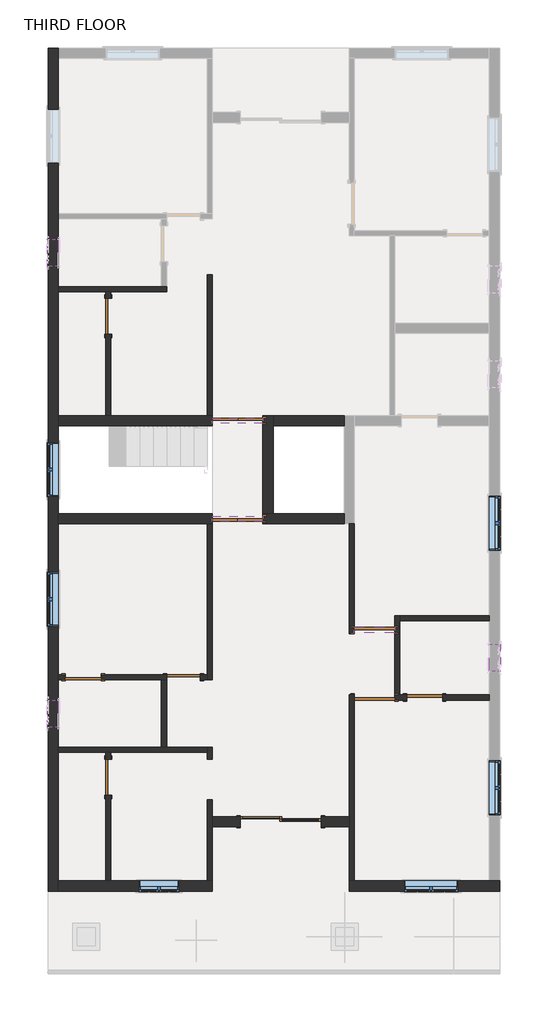
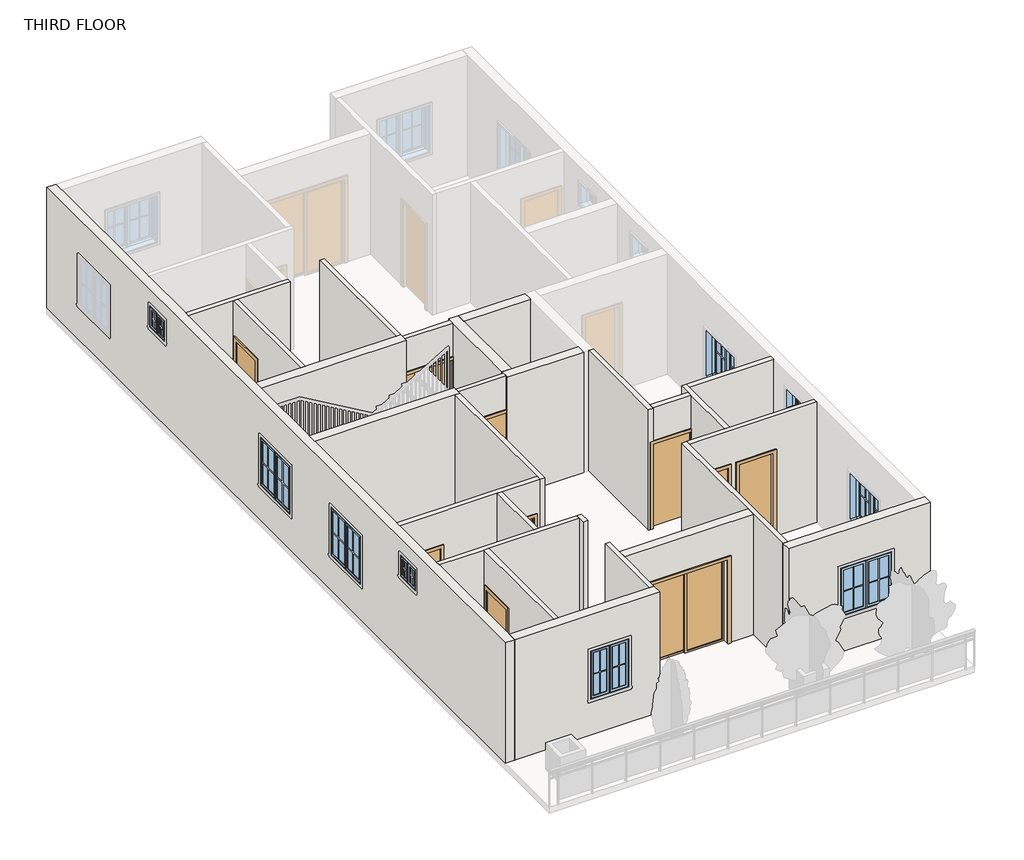
# One storey, part 1 of 4: 27 walls, 10 doors, 9 windows.
"""IFC4 building model written with IfcOpenShell, lengths in millimetres."""

from ifc_helpers import new_model, si_unit, frame, origin, place, context, project, spatial, polyline, outline, extrude, faceted_brep, transform, mapped, element, save
from components import door_31bd1cdd, door_d4d75d1e, door_214872d5, door_d141acb4, door_38851409, single_flush_3_x7_e5f9f3c4, single_flush_3_x7_305aa2a5, window_79894727, window_casement_double_3_x4_d341e8ac, window_casement_double_4_x4_af3140d2

model = new_model("IFC4")

# Units and contexts
model_context = context("Model", 3, world=origin())
ifc_project = project(units=[si_unit("LENGTHUNIT", "METRE", prefix="MILLI")], contexts=[model_context])

# Site, building, storey
site = spatial("IfcSite", under=ifc_project)
building = spatial("IfcBuilding", under=site)
storey = spatial("IfcBuildingStorey", under=building, Name="THIRD FLOOR", Elevation=9601.2)

# Doors
placement = place(None, origin())
door_shape = door_31bd1cdd(model_context)
element("IfcDoor", 1, ObjectType="Door-Double-Flush_Panel : 3'9\"X7'", at=placement, inside=storey, context=model_context, shape_type="MappedRepresentation", body=[
    mapped(door_shape, transform((-2091.0289041, 1664.1153263, 9601.2), x_axis=(1.0, 0.0, 0.0), y_axis=(0.0, 1.0, 0.0), z_axis=(0.0, 0.0, 1.0))),
])
element("IfcDoor", 2, ObjectType="Door-Double-Flush_Panel : 3'9\"X7'", at=placement, inside=storey, context=model_context, shape_type="MappedRepresentation", body=[
    mapped(door_shape, transform((-2091.0289041, -545.7007836, 9601.2), x_axis=(-1.0, 0.0, 0.0), y_axis=(0.0, -1.0, 0.0), z_axis=(0.0, 0.0, 1.0))),
])
door_2_shape = door_d4d75d1e(model_context)
element("IfcDoor", 3, ObjectType="Door-Double-Sliding : 72\" x 84\"", at=placement, inside=storey, context=model_context, shape_type="MappedRepresentation", body=[
    mapped(door_2_shape, transform((-1119.4789041, -7505.2846737, 9601.2), x_axis=(1.0, 0.0, 0.0), y_axis=(0.0, 1.0, 0.0), z_axis=(0.0, 0.0, 1.0))),
])
door_3_shape = door_214872d5(model_context)
element("IfcDoor", 4, ObjectType="Single-Flush : 2'6\"X7'", at=placement, inside=storey, context=model_context, shape_type="MappedRepresentation", body=[
    mapped(door_3_shape, transform((-3310.2289041, -4120.7346737, 9601.2), x_axis=(1.0, 0.0, 0.0), y_axis=(0.0, 1.0, 0.0), z_axis=(0.0, 0.0, 1.0))),
])
door_4_shape = door_d141acb4(model_context)
element("IfcDoor", 5, ObjectType="Single-Flush : 2'8\"X7'", at=placement, inside=storey, context=model_context, shape_type="MappedRepresentation", body=[
    mapped(door_4_shape, transform((-5005.6789041, 4013.6153263, 9601.2), x_axis=(0.0, 1.0, 0.0), y_axis=(-1.0, 0.0, 0.0), z_axis=(0.0, 0.0, 1.0))),
])
element("IfcDoor", 6, ObjectType="Single-Flush : 2'8\"X7'", at=placement, inside=storey, context=model_context, shape_type="MappedRepresentation", body=[
    mapped(door_4_shape, transform((-5570.8289041, -4120.7346737, 9601.2), x_axis=(-1.0, 0.0, 0.0), y_axis=(0.0, -1.0, 0.0), z_axis=(0.0, 0.0, 1.0))),
])
element("IfcDoor", 7, ObjectType="Single-Flush : 2'8\"X7'", at=placement, inside=storey, context=model_context, shape_type="MappedRepresentation", body=[
    mapped(door_4_shape, transform((-5005.6789041, -6374.9846737, 9601.2), x_axis=(0.0, 1.0, 0.0), y_axis=(-1.0, 0.0, 0.0), z_axis=(0.0, 0.0, 1.0))),
])
door_5_shape = door_38851409(model_context)
element("IfcDoor", 8, ObjectType="Single-Flush : 2'8\"X7'", at=placement, inside=storey, context=model_context, shape_type="MappedRepresentation", body=[
    mapped(door_5_shape, transform((2125.3710959, -4577.9346737, 9601.2), x_axis=(-1.0, 0.0, 0.0), y_axis=(0.0, -1.0, 0.0), z_axis=(0.0, 0.0, 1.0))),
])
single_flush_3_x7_shape = single_flush_3_x7_e5f9f3c4(model_context)
element("IfcDoor", 9, ObjectType="Single-Flush : 3'X7'", at=placement, inside=storey, context=model_context, shape_type="MappedRepresentation", body=[
    mapped(single_flush_3_x7_shape, transform((995.0710959, -4577.9346737, 9601.2), x_axis=(-1.0, 0.0, 0.0), y_axis=(0.0, -1.0, 0.0), z_axis=(0.0, 0.0, 1.0))),
])
single_flush_3_x7_2_shape = single_flush_3_x7_305aa2a5(model_context)
element("IfcDoor", 10, ObjectType="Single-Flush : 3'X7'", at=placement, inside=storey, context=model_context, shape_type="MappedRepresentation", body=[
    mapped(single_flush_3_x7_2_shape, transform((995.0710959, -3056.3085282, 9601.2), x_axis=(-1.0, 0.0, 0.0), y_axis=(0.0, -1.0, 0.0), z_axis=(0.0, 0.0, 1.0))),
])

# Walls
element("IfcWall", 11, ObjectType="4.5\"", at=placement, inside=storey, context=model_context, shape_type="Brep", body=[
    faceted_brep([(-6129.6289041, 4572.4153263, 9601.2), (-5062.8289041, 4572.4153263, 9601.2), (-4948.5289041, 4572.4153263, 9601.2), (-3691.2289041, 4572.4153263, 9601.2), (-3691.2289041, 4572.4153263, 12649.2), (-4948.5289041, 4572.4153263, 12649.2), (-5062.8289041, 4572.4153263, 12649.2), (-6129.6289041, 4572.4153263, 12649.2), (-6129.6289041, 4686.7153263, 9601.2), (-6129.6289041, 4686.7153263, 12649.2), (-3805.5289041, 4686.7153263, 12649.2), (-3691.2289041, 4686.7153263, 12649.2), (-3691.2289041, 4686.7153263, 9601.2), (-3805.5289041, 4686.7153263, 9601.2)], [[[0, 1, 2, 3, 4, 5, 6, 7]], [[8, 9, 10, 11, 12, 13]], [[3, 2, 1, 0, 8, 13, 12]], [[7, 6, 5, 4, 11, 10, 9]], [[0, 7, 9, 8]], [[4, 3, 12, 11]]]),
])
element("IfcWall", 12, ObjectType="4.5\"", at=placement, inside=storey, context=model_context, shape_type="SweptSolid", body=[
    extrude(outline(polyline([(4572.4153263, 9601.2), (4420.0153263, 9601.2), (4420.0153263, 11734.8), (3607.2153263, 11734.8), (3607.2153263, 9601.2), (1778.4153263, 9601.2), (1778.4153263, 12649.2), (4572.4153263, 12649.2), (4572.4153263, 9601.2)])), frame((-5062.8289041, 0.0, 0.0), z_axis=(1.0, 0.0, 0.0), x_axis=(0.0, 1.0, 0.0)), (0.0, 0.0, 1.0), 114.3),
])
element("IfcWall", 13, ObjectType="4.5\"", at=placement, inside=storey, context=model_context, shape_type="SweptSolid", body=[
    extrude(outline(polyline([(-2776.8289041, 1778.4153263), (-2776.8289041, 4948.2268555), (-2662.5289041, 4948.2268555), (-2662.5289041, 1778.4153263), (-2776.8289041, 1778.4153263)])), frame((0.0, 0.0, 9601.2), z_axis=(0.0, 0.0, 1.0), x_axis=(1.0, 0.0, 0.0)), (0.0, 0.0, 1.0), 3048.0),
])
element("IfcWall", 14, ObjectType="4.5\"", at=placement, inside=storey, context=model_context, shape_type="Brep", body=[
    faceted_brep([(-2776.8289041, -659.9846737, 9601.2), (-2776.8289041, -4063.5846737, 9601.2), (-2776.8289041, -4177.8846737, 9601.2), (-2776.8289041, -4177.8846737, 12649.2), (-2776.8289041, -4063.5846737, 12649.2), (-2776.8289041, -659.9846737, 12649.2), (-2662.5289041, -659.9846737, 9601.2), (-2662.5289041, -659.9846737, 12649.2), (-2662.5289041, -4177.8846737, 12649.2), (-2662.5289041, -4177.8846737, 9601.2)], [[[0, 1, 2, 3, 4, 5]], [[6, 7, 8, 9]], [[2, 1, 0, 6, 9]], [[5, 4, 3, 8, 7]], [[0, 5, 7, 6]], [[3, 2, 9, 8]]]),
])
element("IfcWall", 15, ObjectType="4.5\"", at=placement, inside=storey, context=model_context, shape_type="Brep", body=[
    faceted_brep([(-2776.8289041, -4063.5846737, 9601.2), (-2929.2289041, -4063.5846737, 9601.2), (-2929.2289041, -4063.5846737, 11734.8), (-3691.2289041, -4063.5846737, 11734.8), (-3691.2289041, -4063.5846737, 9601.2), (-5164.4289041, -4063.5846737, 9601.2), (-5164.4289041, -4063.5846737, 11734.8), (-5977.2289041, -4063.5846737, 11734.8), (-5977.2289041, -4063.5846737, 9601.2), (-6129.6289041, -4063.5846737, 9601.2), (-6129.6289041, -4063.5846737, 12649.2), (-2776.8289041, -4063.5846737, 12649.2), (-2929.2289041, -4177.8846737, 11734.8), (-2929.2289041, -4177.8846737, 9601.2), (-2776.8289041, -4177.8846737, 9601.2), (-2776.8289041, -4177.8846737, 12649.2), (-3691.2289041, -4177.8846737, 12649.2), (-3805.5289041, -4177.8846737, 12649.2), (-6129.6289041, -4177.8846737, 12649.2), (-6129.6289041, -4177.8846737, 9601.2), (-5977.2289041, -4177.8846737, 9601.2), (-5977.2289041, -4177.8846737, 11734.8), (-5164.4289041, -4177.8846737, 11734.8), (-5164.4289041, -4177.8846737, 9601.2), (-3805.5289041, -4177.8846737, 9601.2), (-3691.2289041, -4177.8846737, 9601.2), (-3691.2289041, -4177.8846737, 11734.8)], [[[0, 1, 2, 3, 4, 5, 6, 7, 8, 9, 10, 11]], [[12, 13, 14, 15, 16, 17, 18, 19, 20, 21, 22, 23, 24, 25, 26]], [[9, 8, 20, 19]], [[14, 13, 1, 0]], [[25, 24, 23, 5, 4]], [[11, 10, 18, 17, 16, 15]], [[0, 11, 15, 14]], [[10, 9, 19, 18]], [[21, 20, 8, 7]], [[22, 21, 7, 6]], [[23, 22, 6, 5]], [[2, 1, 13, 12]], [[3, 2, 12, 26]], [[4, 3, 26, 25]]]),
])
element("IfcWall", 16, ObjectType="4.5\"", at=placement, inside=storey, context=model_context, shape_type="Brep", body=[
    faceted_brep([(-3805.5289041, -4177.8846737, 9601.2), (-3805.5289041, -5701.8846737, 9601.2), (-3805.5289041, -5701.8846737, 12649.2), (-3805.5289041, -4177.8846737, 12649.2), (-3691.2289041, -4177.8846737, 9601.2), (-3691.2289041, -4177.8846737, 11734.8), (-3691.2289041, -4177.8846737, 12649.2), (-3691.2289041, -5701.8846737, 12649.2), (-3691.2289041, -5701.8846737, 9601.2)], [[[0, 1, 2, 3]], [[4, 5, 6, 7, 8]], [[1, 0, 4, 8]], [[3, 2, 7, 6]], [[0, 3, 6, 5, 4]], [[2, 1, 8, 7]]]),
])
element("IfcWall", 17, ObjectType="4.5\"", at=placement, inside=storey, context=model_context, shape_type="Brep", body=[
    faceted_brep([(-6129.6289041, -5816.1846737, 9601.2), (-5062.8289041, -5816.1846737, 9601.2), (-4948.5289041, -5816.1846737, 9601.2), (-2776.8289041, -5816.1846737, 9601.2), (-2776.8289041, -5816.1846737, 12649.2), (-4948.5289041, -5816.1846737, 12649.2), (-5062.8289041, -5816.1846737, 12649.2), (-6129.6289041, -5816.1846737, 12649.2), (-6129.6289041, -5701.8846737, 9601.2), (-6129.6289041, -5701.8846737, 12649.2), (-3805.5289041, -5701.8846737, 12649.2), (-3691.2289041, -5701.8846737, 12649.2), (-2776.8289041, -5701.8846737, 12649.2), (-2776.8289041, -5701.8846737, 9601.2), (-3691.2289041, -5701.8846737, 9601.2), (-3805.5289041, -5701.8846737, 9601.2)], [[[0, 1, 2, 3, 4, 5, 6, 7]], [[8, 9, 10, 11, 12, 13, 14, 15]], [[3, 2, 1, 0, 8, 15, 14, 13]], [[7, 6, 5, 4, 12, 11, 10, 9]], [[0, 7, 9, 8]], [[4, 3, 13, 12]]]),
])
element("IfcWall", 18, ObjectType="4.5\"", at=placement, inside=storey, context=model_context, shape_type="Brep", body=[
    faceted_brep([(-2776.8289041, -5701.8846737, 9601.2), (-2776.8289041, -5816.1846737, 9601.2), (-2776.8289041, -5968.5846737, 9601.2), (-2776.8289041, -5968.5846737, 12649.2), (-2776.8289041, -5816.1846737, 12649.2), (-2776.8289041, -5701.8846737, 12649.2), (-2662.5289041, -5701.8846737, 9601.2), (-2662.5289041, -5701.8846737, 12649.2), (-2662.5289041, -5968.5846737, 12649.2), (-2662.5289041, -5968.5846737, 9601.2)], [[[0, 1, 2, 3, 4, 5]], [[6, 7, 8, 9]], [[2, 1, 0, 6, 9]], [[3, 2, 9, 8]], [[5, 4, 3, 8, 7]], [[0, 5, 7, 6]]]),
])
element("IfcWall", 19, ObjectType="4.5\"", at=placement, inside=storey, context=model_context, shape_type="SweptSolid", body=[
    extrude(outline(polyline([(-5816.1846737, 9601.2), (-5968.5846737, 9601.2), (-5968.5846737, 11734.8), (-6781.3846737, 11734.8), (-6781.3846737, 9601.2), (-8711.7846737, 9601.2), (-8711.7846737, 12649.2), (-5816.1846737, 12649.2), (-5816.1846737, 9601.2)])), frame((-5062.8289041, 0.0, 0.0), z_axis=(1.0, 0.0, 0.0), x_axis=(0.0, 1.0, 0.0)), (0.0, 0.0, 1.0), 114.3),
])
element("IfcWall", 20, ObjectType="4.5\"", at=placement, inside=storey, context=model_context, shape_type="Brep", body=[
    faceted_brep([(-2776.8289041, -6882.9846737, 9601.2), (-2776.8289041, -8711.7846737, 9601.2), (-2776.8289041, -8711.7846737, 12649.2), (-2776.8289041, -6882.9846737, 12649.2), (-2662.5289041, -6882.9846737, 9601.2), (-2662.5289041, -6882.9846737, 12649.2), (-2662.5289041, -7263.9846737, 12649.2), (-2662.5289041, -7492.5846737, 12649.2), (-2662.5289041, -8711.7846737, 12649.2), (-2662.5289041, -8711.7846737, 9601.2), (-2662.5289041, -7492.5846737, 9601.2), (-2662.5289041, -7263.9846737, 9601.2)], [[[0, 1, 2, 3]], [[4, 5, 6, 7, 8, 9, 10, 11]], [[1, 0, 4, 11, 10, 9]], [[3, 2, 8, 7, 6, 5]], [[0, 3, 5, 4]], [[2, 1, 9, 8]]]),
])
element("IfcWall", 21, ObjectType="4.5\"", at=placement, inside=storey, context=model_context, shape_type="Brep", body=[
    faceted_brep([(423.5710959, -659.9846737, 9601.2), (423.5710959, -3136.3185282, 9601.2), (423.5710959, -3136.3185282, 12649.2), (423.5710959, -659.9846737, 12649.2), (537.8710959, -659.9846737, 9601.2), (537.8710959, -659.9846737, 12649.2), (537.8710959, -2999.1585282, 12649.2), (537.8710959, -3113.4585282, 12649.2), (537.8710959, -3136.3185282, 12649.2), (537.8710959, -3136.3185282, 9601.2), (537.8710959, -3113.4585282, 9601.2), (537.8710959, -2999.1585282, 9601.2)], [[[0, 1, 2, 3]], [[4, 5, 6, 7, 8, 9, 10, 11]], [[1, 0, 4, 11, 10, 9]], [[2, 1, 9, 8]], [[3, 2, 8, 7, 6, 5]], [[0, 3, 5, 4]]]),
])
element("IfcWall", 22, ObjectType="4.5\"", at=placement, inside=storey, context=model_context, shape_type="Brep", body=[
    faceted_brep([(423.5710959, -4520.7846737, 9601.2), (423.5710959, -7263.9846737, 9601.2), (423.5710959, -7492.5846737, 9601.2), (423.5710959, -8711.7846737, 9601.2), (423.5710959, -8711.7846737, 12649.2), (423.5710959, -7492.5846737, 12649.2), (423.5710959, -7263.9846737, 12649.2), (423.5710959, -4520.7846737, 12649.2), (537.8710959, -4520.7846737, 9601.2), (537.8710959, -4520.7846737, 11734.8), (537.8710959, -4520.7846737, 12649.2), (537.8710959, -4635.0846737, 12649.2), (537.8710959, -8711.7846737, 12649.2), (537.8710959, -8711.7846737, 9601.2)], [[[0, 1, 2, 3, 4, 5, 6, 7]], [[8, 9, 10, 11, 12, 13]], [[3, 2, 1, 0, 8, 13]], [[7, 6, 5, 4, 12, 11, 10]], [[4, 3, 13, 12]], [[0, 7, 10, 9, 8]]]),
])
element("IfcWall", 23, ObjectType="4.5\"", at=placement, inside=storey, context=model_context, shape_type="Brep", body=[
    faceted_brep([(1718.9710959, -4520.7846737, 11734.8), (1718.9710959, -4520.7846737, 9601.2), (1566.5710959, -4520.7846737, 9601.2), (1452.2710959, -4520.7846737, 9601.2), (1452.2710959, -4520.7846737, 11734.8), (537.8710959, -4520.7846737, 11734.8), (537.8710959, -4520.7846737, 12649.2), (1452.2710959, -4520.7846737, 12649.2), (1566.5710959, -4520.7846737, 12649.2), (3585.8710959, -4520.7846737, 12649.2), (3585.8710959, -4520.7846737, 9601.2), (2531.7710959, -4520.7846737, 9601.2), (2531.7710959, -4520.7846737, 11734.8), (1452.2710959, -4635.0846737, 9601.2), (1718.9710959, -4635.0846737, 9601.2), (1718.9710959, -4635.0846737, 11734.8), (2531.7710959, -4635.0846737, 11734.8), (2531.7710959, -4635.0846737, 9601.2), (3585.8710959, -4635.0846737, 9601.2), (3585.8710959, -4635.0846737, 12649.2), (537.8710959, -4635.0846737, 12649.2), (537.8710959, -4635.0846737, 11734.8), (1452.2710959, -4635.0846737, 11734.8)], [[[0, 1, 2, 3, 4, 5, 6, 7, 8, 9, 10, 11, 12]], [[13, 14, 15, 16, 17, 18, 19, 20, 21, 22]], [[11, 10, 18, 17]], [[3, 2, 1, 14, 13]], [[9, 8, 7, 6, 20, 19]], [[10, 9, 19, 18]], [[20, 6, 5, 21]], [[4, 22, 21, 5]], [[22, 4, 3, 13]], [[15, 14, 1, 0]], [[16, 15, 0, 12]], [[17, 16, 12, 11]]]),
])
element("IfcWall", 24, ObjectType="4.5\"", at=placement, inside=storey, context=model_context, shape_type="Brep", body=[
    faceted_brep([(1566.5710959, -4520.7846737, 9601.2), (1566.5710959, -2844.3846737, 9601.2), (1566.5710959, -2730.0846737, 9601.2), (1566.5710959, -2730.0846737, 12649.2), (1566.5710959, -2844.3846737, 12649.2), (1566.5710959, -4520.7846737, 12649.2), (1452.2710959, -4520.7846737, 9601.2), (1452.2710959, -4520.7846737, 11734.8), (1452.2710959, -4520.7846737, 12649.2), (1452.2710959, -3113.4585282, 12649.2), (1452.2710959, -2999.1585282, 12649.2), (1452.2710959, -2730.0846737, 12649.2), (1452.2710959, -2730.0846737, 9601.2), (1452.2710959, -2999.1585282, 9601.2), (1452.2710959, -3113.4585282, 9601.2)], [[[0, 1, 2, 3, 4, 5]], [[6, 7, 8, 9, 10, 11, 12, 13, 14]], [[2, 1, 0, 6, 14, 13, 12]], [[5, 4, 3, 11, 10, 9, 8]], [[0, 5, 8, 7, 6]], [[3, 2, 12, 11]]]),
])
element("IfcWall", 25, ObjectType="4.5\"", at=placement, inside=storey, context=model_context, shape_type="SweptSolid", body=[
    extrude(outline(polyline([(3585.8710959, -2844.3846737), (1566.5710959, -2844.3846737), (1566.5710959, -2730.0846737), (3585.8710959, -2730.0846737), (3585.8710959, -2844.3846737)])), frame((0.0, 0.0, 9601.2), z_axis=(0.0, 0.0, 1.0), x_axis=(1.0, 0.0, 0.0)), (0.0, 0.0, 1.0), 3048.0),
])
element("IfcWall", 26, ObjectType="4.5\"", at=placement, inside=storey, context=model_context, shape_type="SweptSolid", body=[
    extrude(outline(polyline([(-1519.5289041, 1606.9653263), (-2662.5289041, 1606.9653263), (-2662.5289041, 1721.2653263), (-1519.5289041, 1721.2653263), (-1519.5289041, 1606.9653263)])), frame((0.0, 0.0, 11734.8), z_axis=(0.0, 0.0, 1.0), x_axis=(1.0, 0.0, 0.0)), (0.0, 0.0, 1.0), 914.4),
])
element("IfcWall", 27, ObjectType="4.5\"", at=placement, inside=storey, context=model_context, shape_type="SweptSolid", body=[
    extrude(outline(polyline([(-1519.5289041, -602.8507836), (-2662.5289041, -602.8507836), (-2662.5289041, -488.5507836), (-1519.5289041, -488.5507836), (-1519.5289041, -602.8507836)])), frame((0.0, 0.0, 11734.8), z_axis=(0.0, 0.0, 1.0), x_axis=(1.0, 0.0, 0.0)), (0.0, 0.0, 1.0), 914.4),
])
element("IfcWall", 28, ObjectType="4.5\"", at=placement, inside=storey, context=model_context, shape_type="SweptSolid", body=[
    extrude(outline(polyline([(1452.2710959, -3113.4585282), (537.8710959, -3113.4585282), (537.8710959, -2999.1585282), (1452.2710959, -2999.1585282), (1452.2710959, -3113.4585282)])), frame((0.0, 0.0, 11734.8), z_axis=(0.0, 0.0, 1.0), x_axis=(1.0, 0.0, 0.0)), (0.0, 0.0, 1.0), 914.4),
])
element("IfcWall", 29, ObjectType="9\"", at=placement, inside=storey, context=model_context, shape_type="Brep", body=[
    faceted_brep([(-6358.2289041, 10058.8153263, 9601.2), (-6358.2289041, -8940.3846737, 9601.2), (-6358.2289041, -8940.3846737, 12649.2), (-6358.2289041, 10058.8153263, 12649.2), (-6358.2289041, 8687.2153263, 11734.8), (-6358.2289041, 7468.0153263, 11734.8), (-6358.2289041, 7468.0153263, 10515.6), (-6358.2289041, 8687.2153263, 10515.6), (-6358.2289041, -1752.1846737, 11734.8), (-6358.2289041, -2971.3846737, 11734.8), (-6358.2289041, -2971.3846737, 10515.6), (-6358.2289041, -1752.1846737, 10515.6), (-6358.2289041, 1168.8153263, 11734.8), (-6358.2289041, -50.3846737, 11734.8), (-6358.2289041, -50.3846737, 10515.6), (-6358.2289041, 1168.8153263, 10515.6), (-6358.2289041, 5753.5153263, 12268.2), (-6358.2289041, 5143.9153263, 12268.2), (-6358.2289041, 5143.9153263, 11734.8), (-6358.2289041, 5753.5153263, 11734.8), (-6358.2289041, -4635.0846737, 12268.2), (-6358.2289041, -5244.6846737, 12268.2), (-6358.2289041, -5244.6846737, 11734.8), (-6358.2289041, -4635.0846737, 11734.8), (-6129.6289041, 10058.8153263, 9601.2), (-6129.6289041, 10058.8153263, 12649.2), (-6129.6289041, 9830.2153263, 12649.2), (-6129.6289041, 6325.0153263, 12649.2), (-6129.6289041, 6210.7153263, 12649.2), (-6129.6289041, 4686.7153263, 12649.2), (-6129.6289041, 4572.4153263, 12649.2), (-6129.6289041, 1778.4153263, 12649.2), (-6129.6289041, 1549.8153263, 12649.2), (-6129.6289041, -431.3846737, 12649.2), (-6129.6289041, -659.9846737, 12649.2), (-6129.6289041, -4063.5846737, 12649.2), (-6129.6289041, -4177.8846737, 12649.2), (-6129.6289041, -5701.8846737, 12649.2), (-6129.6289041, -5816.1846737, 12649.2), (-6129.6289041, -8711.7846737, 12649.2), (-6129.6289041, -8940.3846737, 12649.2), (-6129.6289041, -8940.3846737, 9601.2), (-6129.6289041, -8711.7846737, 9601.2), (-6129.6289041, -5816.1846737, 9601.2), (-6129.6289041, -5701.8846737, 9601.2), (-6129.6289041, -4177.8846737, 9601.2), (-6129.6289041, -4063.5846737, 9601.2), (-6129.6289041, -659.9846737, 9601.2), (-6129.6289041, -431.3846737, 9601.2), (-6129.6289041, 1549.8153263, 9601.2), (-6129.6289041, 1778.4153263, 9601.2), (-6129.6289041, 4572.4153263, 9601.2), (-6129.6289041, 4686.7153263, 9601.2), (-6129.6289041, 6210.7153263, 9601.2), (-6129.6289041, 6325.0153263, 9601.2), (-6129.6289041, 9830.2153263, 9601.2), (-6129.6289041, 8687.2153263, 11734.8), (-6129.6289041, 8687.2153263, 10515.6), (-6129.6289041, 7468.0153263, 10515.6), (-6129.6289041, 7468.0153263, 11734.8), (-6129.6289041, -1752.1846737, 11734.8), (-6129.6289041, -1752.1846737, 10515.6), (-6129.6289041, -2971.3846737, 10515.6), (-6129.6289041, -2971.3846737, 11734.8), (-6129.6289041, 1168.8153263, 11734.8), (-6129.6289041, 1168.8153263, 10515.6), (-6129.6289041, -50.3846737, 10515.6), (-6129.6289041, -50.3846737, 11734.8), (-6129.6289041, 5753.5153263, 12268.2), (-6129.6289041, 5753.5153263, 11734.8), (-6129.6289041, 5143.9153263, 11734.8), (-6129.6289041, 5143.9153263, 12268.2), (-6129.6289041, -4635.0846737, 12268.2), (-6129.6289041, -4635.0846737, 11734.8), (-6129.6289041, -5244.6846737, 11734.8), (-6129.6289041, -5244.6846737, 12268.2)], [[[0, 1, 2, 3], [4, 5, 6, 7], [8, 9, 10, 11], [12, 13, 14, 15], [16, 17, 18, 19], [20, 21, 22, 23]], [[24, 25, 26, 27, 28, 29, 30, 31, 32, 33, 34, 35, 36, 37, 38, 39, 40, 41, 42, 43, 44, 45, 46, 47, 48, 49, 50, 51, 52, 53, 54, 55], [56, 57, 58, 59], [60, 61, 62, 63], [64, 65, 66, 67], [68, 69, 70, 71], [72, 73, 74, 75]], [[1, 0, 24, 55, 54, 53, 52, 51, 50, 49, 48, 47, 46, 45, 44, 43, 42, 41]], [[3, 2, 40, 39, 38, 37, 36, 35, 34, 33, 32, 31, 30, 29, 28, 27, 26, 25]], [[2, 1, 41, 40]], [[0, 3, 25, 24]], [[57, 56, 4, 7]], [[58, 57, 7, 6]], [[59, 58, 6, 5]], [[56, 59, 5, 4]], [[61, 60, 8, 11]], [[62, 61, 11, 10]], [[63, 62, 10, 9]], [[60, 63, 9, 8]], [[65, 64, 12, 15]], [[66, 65, 15, 14]], [[67, 66, 14, 13]], [[64, 67, 13, 12]], [[69, 68, 16, 19]], [[70, 69, 19, 18]], [[71, 70, 18, 17]], [[68, 71, 17, 16]], [[73, 72, 20, 23]], [[74, 73, 23, 22]], [[75, 74, 22, 21]], [[72, 75, 21, 20]]]),
])
element("IfcWall", 30, ObjectType="9\"", at=placement, inside=storey, context=model_context, shape_type="Brep", body=[
    faceted_brep([(-6129.6289041, -8940.3846737, 9601.2), (-2662.5289041, -8940.3846737, 9601.2), (-2662.5289041, -8940.3846737, 12649.2), (-6129.6289041, -8940.3846737, 12649.2), (-4319.8789041, -8940.3846737, 11734.8), (-3405.4789041, -8940.3846737, 11734.8), (-3405.4789041, -8940.3846737, 10515.6), (-4319.8789041, -8940.3846737, 10515.6), (-6129.6289041, -8711.7846737, 9601.2), (-6129.6289041, -8711.7846737, 12649.2), (-5062.8289041, -8711.7846737, 12649.2), (-4948.5289041, -8711.7846737, 12649.2), (-2776.8289041, -8711.7846737, 12649.2), (-2662.5289041, -8711.7846737, 12649.2), (-2662.5289041, -8711.7846737, 9601.2), (-2776.8289041, -8711.7846737, 9601.2), (-4948.5289041, -8711.7846737, 9601.2), (-5062.8289041, -8711.7846737, 9601.2), (-4319.8789041, -8711.7846737, 11734.8), (-4319.8789041, -8711.7846737, 10515.6), (-3405.4789041, -8711.7846737, 10515.6), (-3405.4789041, -8711.7846737, 11734.8)], [[[0, 1, 2, 3], [4, 5, 6, 7]], [[8, 9, 10, 11, 12, 13, 14, 15, 16, 17], [18, 19, 20, 21]], [[1, 0, 8, 17, 16, 15, 14]], [[3, 2, 13, 12, 11, 10, 9]], [[0, 3, 9, 8]], [[2, 1, 14, 13]], [[19, 18, 4, 7]], [[20, 19, 7, 6]], [[21, 20, 6, 5]], [[18, 21, 5, 4]]]),
])
element("IfcWall", 31, ObjectType="9\"", at=placement, inside=storey, context=model_context, shape_type="Brep", body=[
    faceted_brep([(423.5710959, -8940.3846737, 9601.2), (3814.4710959, -8940.3846737, 9601.2), (3814.4710959, -8940.3846737, 12649.2), (423.5710959, -8940.3846737, 12649.2), (1662.2107801, -8940.3846737, 11734.8), (2881.4107801, -8940.3846737, 11734.8), (2881.4107801, -8940.3846737, 10515.6), (1662.2107801, -8940.3846737, 10515.6), (423.5710959, -8711.7846737, 9601.2), (423.5710959, -8711.7846737, 12649.2), (537.8710959, -8711.7846737, 12649.2), (3585.8710959, -8711.7846737, 12649.2), (3814.4710959, -8711.7846737, 12649.2), (3814.4710959, -8711.7846737, 9601.2), (3585.8710959, -8711.7846737, 9601.2), (537.8710959, -8711.7846737, 9601.2), (1662.2107801, -8711.7846737, 11734.8), (1662.2107801, -8711.7846737, 10515.6), (2881.4107801, -8711.7846737, 10515.6), (2881.4107801, -8711.7846737, 11734.8)], [[[0, 1, 2, 3], [4, 5, 6, 7]], [[8, 9, 10, 11, 12, 13, 14, 15], [16, 17, 18, 19]], [[1, 0, 8, 15, 14, 13]], [[3, 2, 12, 11, 10, 9]], [[2, 1, 13, 12]], [[0, 3, 9, 8]], [[17, 16, 4, 7]], [[18, 17, 7, 6]], [[19, 18, 6, 5]], [[16, 19, 5, 4]]]),
])
element("IfcWall", 32, ObjectType="9\"", at=placement, inside=storey, context=model_context, shape_type="Brep", body=[
    faceted_brep([(-6129.6289041, 1549.8153263, 9601.2), (-2662.5289041, 1549.8153263, 9601.2), (-2662.5289041, 1549.8153263, 12649.2), (-6129.6289041, 1549.8153263, 12649.2), (-6129.6289041, 1778.4153263, 9601.2), (-6129.6289041, 1778.4153263, 12649.2), (-5062.8289041, 1778.4153263, 12649.2), (-4948.5289041, 1778.4153263, 12649.2), (-2776.8289041, 1778.4153263, 12649.2), (-2662.5289041, 1778.4153263, 12649.2), (-2662.5289041, 1778.4153263, 9601.2), (-2776.8289041, 1778.4153263, 9601.2), (-4948.5289041, 1778.4153263, 9601.2), (-5062.8289041, 1778.4153263, 9601.2), (-2662.5289041, 1606.9653263, 12649.2), (-2662.5289041, 1721.2653263, 12649.2)], [[[0, 1, 2, 3]], [[4, 5, 6, 7, 8, 9, 10, 11, 12, 13]], [[1, 0, 4, 13, 12, 11, 10]], [[3, 2, 14, 15, 9, 8, 7, 6, 5]], [[0, 3, 5, 4]], [[2, 1, 10, 9, 15, 14]]]),
])
element("IfcWall", 33, ObjectType="9\"", at=placement, inside=storey, context=model_context, shape_type="Brep", body=[
    faceted_brep([(-6129.6289041, -659.9846737, 9601.2), (-2776.8289041, -659.9846737, 9601.2), (-2662.5289041, -659.9846737, 9601.2), (-2662.5289041, -659.9846737, 12649.2), (-2776.8289041, -659.9846737, 12649.2), (-6129.6289041, -659.9846737, 12649.2), (-6129.6289041, -431.3846737, 9601.2), (-6129.6289041, -431.3846737, 12649.2), (-2662.5289041, -431.3846737, 12649.2), (-2662.5289041, -431.3846737, 9601.2), (-2662.5289041, -602.8507836, 12649.2), (-2662.5289041, -488.5507836, 12649.2)], [[[0, 1, 2, 3, 4, 5]], [[6, 7, 8, 9]], [[2, 1, 0, 6, 9]], [[5, 4, 3, 10, 11, 8, 7]], [[0, 5, 7, 6]], [[3, 2, 9, 8, 11, 10]]]),
])
element("IfcWall", 34, ObjectType="9\"", at=placement, inside=storey, context=model_context, shape_type="Brep", body=[
    faceted_brep([(309.2710959, -431.3846737, 9601.2), (-1290.9289041, -431.3846737, 9601.2), (-1519.5289041, -431.3846737, 9601.2), (-1519.5289041, -431.3846737, 12649.2), (-1290.9289041, -431.3846737, 12649.2), (309.2710959, -431.3846737, 12649.2), (309.2710959, -659.9846737, 9601.2), (309.2710959, -659.9846737, 12649.2), (-1519.5289041, -659.9846737, 12649.2), (-1519.5289041, -659.9846737, 9601.2), (-1519.5289041, -488.5507836, 12649.2), (-1519.5289041, -602.8507836, 12649.2)], [[[0, 1, 2, 3, 4, 5]], [[6, 7, 8, 9]], [[2, 1, 0, 6, 9]], [[5, 4, 3, 10, 11, 8, 7]], [[0, 5, 7, 6]], [[3, 2, 9, 8, 11, 10]]]),
])
element("IfcWall", 35, ObjectType="9\"", at=placement, inside=storey, context=model_context, shape_type="Brep", body=[
    faceted_brep([(-1290.9289041, -431.3846737, 9601.2), (-1290.9289041, 1549.8153263, 9601.2), (-1290.9289041, 1778.4153263, 9601.2), (-1290.9289041, 1778.4153263, 12649.2), (-1290.9289041, 1549.8153263, 12649.2), (-1290.9289041, -431.3846737, 12649.2), (-1519.5289041, -431.3846737, 9601.2), (-1519.5289041, -431.3846737, 12649.2), (-1519.5289041, 1606.9653263, 12649.2), (-1519.5289041, 1721.2653263, 12649.2), (-1519.5289041, 1778.4153263, 12649.2), (-1519.5289041, 1778.4153263, 9601.2)], [[[0, 1, 2, 3, 4, 5]], [[6, 7, 8, 9, 10, 11]], [[2, 1, 0, 6, 11]], [[5, 4, 3, 10, 9, 8, 7]], [[0, 5, 7, 6]], [[3, 2, 11, 10]]]),
])
element("IfcWall", 36, ObjectType="9\"", at=placement, inside=storey, context=model_context, shape_type="SweptSolid", body=[
    extrude(outline(polyline([(-1290.9289041, 1778.4153263), (309.2710959, 1778.4153263), (309.2710959, 1549.8153263), (-1290.9289041, 1549.8153263), (-1290.9289041, 1778.4153263)])), frame((0.0, 0.0, 9601.2), z_axis=(0.0, 0.0, 1.0), x_axis=(1.0, 0.0, 0.0)), (0.0, 0.0, 1.0), 3048.0),
])
element("IfcWall", 37, ObjectType="9\"", at=placement, inside=storey, context=model_context, shape_type="SweptSolid", body=[
    extrude(outline(polyline([(11734.8, -205.0789041), (9601.2, -205.0789041), (9601.2, 423.5710959), (12649.2, 423.5710959), (12649.2, -2662.5289041), (9601.2, -2662.5289041), (9601.2, -2033.8789041), (11734.8, -2033.8789041), (11734.8, -205.0789041)])), frame((0.0, -7492.5846737, 0.0), z_axis=(0.0, 1.0, 0.0), x_axis=(0.0, 0.0, 1.0)), (0.0, 0.0, 1.0), 228.6),
])

# Windows
window_shape = window_79894727(model_context)
element("IfcWindow", 38, ObjectType="Window-Casement-Double : 2'X1'9\"", at=placement, inside=storey, context=model_context, shape_type="MappedRepresentation", body=[
    mapped(window_shape, transform((-6243.9289041, 5448.7153263, 9601.2), x_axis=(0.0, 1.0, 0.0), y_axis=(-1.0, 0.0, 0.0), z_axis=(0.0, 0.0, 1.0))),
])
element("IfcWindow", 39, ObjectType="Window-Casement-Double : 2'X1'9\"", at=placement, inside=storey, context=model_context, shape_type="MappedRepresentation", body=[
    mapped(window_shape, transform((-6243.9289041, -4939.8846737, 9601.2), x_axis=(0.0, 1.0, 0.0), y_axis=(-1.0, 0.0, 0.0), z_axis=(0.0, 0.0, 1.0))),
])
element("IfcWindow", 40, ObjectType="Window-Casement-Double : 2'X1'9\"", at=placement, inside=storey, context=model_context, shape_type="MappedRepresentation", body=[
    mapped(window_shape, transform((3700.1710959, -3682.5846737, 9601.2), x_axis=(0.0, -1.0, 0.0), y_axis=(1.0, 0.0, 0.0), z_axis=(0.0, 0.0, 1.0))),
])
window_casement_double_3_x4_shape = window_casement_double_3_x4_d341e8ac(model_context)
element("IfcWindow", 41, ObjectType="Window-Casement-Double : 3'X4'", at=placement, inside=storey, context=model_context, shape_type="MappedRepresentation", body=[
    mapped(window_casement_double_3_x4_shape, transform((-3862.6789041, -8826.0846737, 9601.2), x_axis=(-1.0, 0.0, 0.0), y_axis=(0.0, -1.0, 0.0), z_axis=(0.0, 0.0, 1.0))),
])
window_casement_double_4_x4_shape = window_casement_double_4_x4_af3140d2(model_context)
element("IfcWindow", 42, ObjectType="Window-Casement-Double : 4'X4'", at=placement, inside=storey, context=model_context, shape_type="MappedRepresentation", body=[
    mapped(window_casement_double_4_x4_shape, transform((-6243.9289041, -2361.7846737, 9601.2), x_axis=(0.0, 1.0, 0.0), y_axis=(-1.0, 0.0, 0.0), z_axis=(0.0, 0.0, 1.0))),
])
element("IfcWindow", 43, ObjectType="Window-Casement-Double : 4'X4'", at=placement, inside=storey, context=model_context, shape_type="MappedRepresentation", body=[
    mapped(window_casement_double_4_x4_shape, transform((2271.8107801, -8826.0846737, 9601.2), x_axis=(-1.0, 0.0, 0.0), y_axis=(0.0, -1.0, 0.0), z_axis=(0.0, 0.0, 1.0))),
])
element("IfcWindow", 44, ObjectType="Window-Casement-Double : 4'X4'", at=placement, inside=storey, context=model_context, shape_type="MappedRepresentation", body=[
    mapped(window_casement_double_4_x4_shape, transform((3700.1710959, -6616.2846737, 9601.2), x_axis=(0.0, -1.0, 0.0), y_axis=(1.0, 0.0, 0.0), z_axis=(0.0, 0.0, 1.0))),
])
element("IfcWindow", 45, ObjectType="Window-Casement-Double : 4'X4'", at=placement, inside=storey, context=model_context, shape_type="MappedRepresentation", body=[
    mapped(window_casement_double_4_x4_shape, transform((3700.1710959, -647.2846737, 9601.2), x_axis=(0.0, -1.0, 0.0), y_axis=(1.0, 0.0, 0.0), z_axis=(0.0, 0.0, 1.0))),
])
element("IfcWindow", 46, ObjectType="Window-Casement-Double : 4'X4'", at=placement, inside=storey, context=model_context, shape_type="MappedRepresentation", body=[
    mapped(window_casement_double_4_x4_shape, transform((-6243.9289041, 559.2153263, 9601.2), x_axis=(0.0, 1.0, 0.0), y_axis=(-1.0, 0.0, 0.0), z_axis=(0.0, 0.0, 1.0))),
])

save(model, "model.ifc")

# Revit data of these elements
# Type "Door-Double-Flush_Panel : 3'9\"X7'"
#   Type Mark = "11"
#   Construction Type Id = "DOOR"
#   Assembly Code = "C1020"
#   Analytic Construction = "Wooden"
#   Thickness = 0' - 2"
#   Thermal Resistance (R) = 2.5876 (h·ft²·°F)/BTU
#   Swing Angle [instance default] = 90.00°
#   Panel Width = 1' - 10 1/2"
#   Heat Transfer Coefficient (U) = 0.3865 BTU/(h·ft²·°F)
#   Height = 7' - 0"
#   Trim Projection Ext = 0' - 1"
#   Trim Projection Int = 0' - 1"
#   Trim Width = 0' - 3"
#   Width = 3' - 9"
#   Define Thermal Properties by = 1
#   Panel Material = Wood - Birch - Solid Stained Light Low Gloss
#   Trim Material = Paint - Sienna
#   Visual Light Transmittance = 0
#   Solar Heat Gain Coefficient = 0
#   Function = (empty or 0)
#   Wall Closure = (empty or 0)
# Type "Door-Double-Sliding : 72\" x 84\""
#   Type Mark = "14"
#   Construction Type Id = "opn-d45"
#   Assembly Code = "C1020"
#   Analytic Construction = "Wood frame, double glass door "
#   Thickness = 0' - 2"
#   Thermal Resistance (R) = 1.8150 (h·ft²·°F)/BTU
#   Heat Transfer Coefficient (U) = 0.5510 BTU/(h·ft²·°F)
#   Height = 7' - 0"
#   Rail Width = 0' - 2"
#   Stiles = 0' - 2"
#   Trim Projection Ext = 0' - 1"
#   Trim Projection Int = 0' - 1"
#   Trim Width = 0' - 3"
#   Width = 6' - 0"
#   Define Thermal Properties by = 1
#   Glazing = Glass
#   Panel Material = Wood - Birch - Solid Stained Light Low Gloss
#   Trim Material = Paint - Sienna
#   Visual Light Transmittance = 0
#   Solar Heat Gain Coefficient = 0
#   Function = (empty or 0)
#   Wall Closure = (empty or 0)
# Type "Single-Flush : 2'6\"X7'"
#   Type Mark = "13"
#   Construction Type Id = "MDOOR"
#   Assembly Code = "C1020"
#   Analytic Construction = "Metal"
#   Thickness = 0' - 2"
#   Heat Transfer Coefficient (U) = 0.651978 BTU/(h·ft²·°F)
#   Height = 7' - 0"
#   Trim Projection Ext = 0' - 1"
#   Trim Projection Int = 0' - 1"
#   Trim Width = 0' - 3"
#   Width = 2' - 6"
#   Define Thermal Properties by = 1
#   Door Material = Door - Panel
#   Frame Material = Door - Frame
#   Visual Light Transmittance = 0
#   Solar Heat Gain Coefficient = 0
#   Function = (empty or 0)
#   Wall Closure = (empty or 0)
# Type "Single-Flush : 2'8\"X7'"
#   Type Mark = "12"
#   Construction Type Id = "MDOOR"
#   Assembly Code = "C1020"
#   Analytic Construction = "Metal"
#   Thickness = 0' - 2"
#   Heat Transfer Coefficient (U) = 0.651978 BTU/(h·ft²·°F)
#   Height = 7' - 0"
#   Trim Projection Ext = 0' - 1"
#   Trim Projection Int = 0' - 1"
#   Trim Width = 0' - 3"
#   Width = 2' - 8"
#   Define Thermal Properties by = 1
#   Door Material = Door - Panel
#   Frame Material = Door - Frame
#   Visual Light Transmittance = 0
#   Solar Heat Gain Coefficient = 0
#   Function = (empty or 0)
#   Wall Closure = (empty or 0)
# Type "Single-Flush : 3'X7'"
#   Type Mark = "8"
#   Construction Type Id = "MDOOR"
#   Assembly Code = "C1020"
#   Analytic Construction = "Metal"
#   Thickness = 0' - 2"
#   Heat Transfer Coefficient (U) = 0.651978 BTU/(h·ft²·°F)
#   Height = 7' - 0"
#   Trim Projection Ext = 0' - 1"
#   Trim Projection Int = 0' - 1"
#   Trim Width = 0' - 3"
#   Width = 3' - 0"
#   Define Thermal Properties by = 1
#   Door Material = Door - Panel
#   Frame Material = Door - Frame
#   Visual Light Transmittance = 0
#   Solar Heat Gain Coefficient = 0
#   Function = (empty or 0)
#   Wall Closure = (empty or 0)
# Type "4.5\""
#   Assembly Code = "B2010"
#   Layers, outside or top first: 0' - 4 1/2" no material (function 1)
# Type "9\""
#   Assembly Code = "B2010"
#   Layers, outside or top first: 0' - 9" "WALL" (function 1)
# Type "Window-Casement-Double : 2'X1'9\""
#   Type Mark = "22"
#   Fire Rating = "0.5h"
#   Assembly Code = "B2020100"
#   Analytic Construction = "Double glazing - domestic"
#   Frame Extension [instance default] = 0' - 0 1/4"
#   Window Inset [instance default] = 0' - 0"
#   Wall Thickness [instance default] = 0' - 6"
#   Interior Wall Closure [instance default] = 0' - 2 1/4"
#   Half Width = 1' - 0"
#   Visual Light Transmittance = 0.81
#   Thermal Resistance (R) = 1.8146 (h·ft²·°F)/BTU
#   Solar Heat Gain Coefficient = 0.76
#   Rough Width = 2' - 0 1/2"
#   Rough Height = 1' - 9 1/2"
#   Height = 1' - 9"
#   Heat Transfer Coefficient (U) = 0.5511 BTU/(h·ft²·°F)
#   Exterior Wall Closure [instance default] = 0' - 1 1/4"
#   Extension Jamb [instance default] = 0' - 2 1/4"
#   Default Sill Height = 7' - 0"
#   Width = 2' - 0"
#   Muntin Visibility = yes
#   Interior Trim Visibility [instance default] = yes
#   Exterior Trim Visibility [instance default] = yes
#   Extension Jamb Visibility [instance default] = yes
#   Interior Trim Material = Wood - Stained
#   Muntin Pattern = Muntin Pattern_2x2 : Muntin Pattern_2x2
#   Interior Trim = Trim-Window-Interior-Flat : Picture Frame
#   Interior Frame Material = Wood - Stained
#   Glass Panel Material = Glass
#   Exterior Trim Material = Clad - White
#   Exterior Trim = Trim-Window-Exterior-Flat : with Sill
#   Exterior Frame Material = Clad - White
#   Wall Closure = (empty or 0)
# Type "Window-Casement-Double : 3'X4'"
#   Type Mark = "21"
#   Fire Rating = "0.5h"
#   Assembly Code = "B2020100"
#   Analytic Construction = "Double glazing - domestic"
#   Frame Extension [instance default] = 0' - 0 1/4"
#   Window Inset [instance default] = 0' - 0"
#   Wall Thickness [instance default] = 0' - 6"
#   Interior Wall Closure [instance default] = 0' - 2 1/4"
#   Half Width = 1' - 6"
#   Visual Light Transmittance = 0.81
#   Thermal Resistance (R) = 1.8146 (h·ft²·°F)/BTU
#   Solar Heat Gain Coefficient = 0.76
#   Rough Width = 3' - 0 1/2"
#   Rough Height = 4' - 0 1/2"
#   Height = 4' - 0"
#   Heat Transfer Coefficient (U) = 0.5511 BTU/(h·ft²·°F)
#   Exterior Wall Closure [instance default] = 0' - 1 1/4"
#   Extension Jamb [instance default] = 0' - 2 1/4"
#   Default Sill Height = 3' - 0"
#   Width = 3' - 0"
#   Muntin Visibility = yes
#   Interior Trim Visibility [instance default] = yes
#   Exterior Trim Visibility [instance default] = yes
#   Extension Jamb Visibility [instance default] = yes
#   Interior Trim Material = Wood - Stained
#   Muntin Pattern = Muntin Pattern_2x2 : Muntin Pattern_2x2
#   Interior Trim = Trim-Window-Interior-Flat : Picture Frame
#   Interior Frame Material = Wood - Stained
#   Glass Panel Material = Glass
#   Exterior Trim Material = Clad - White
#   Exterior Trim = Trim-Window-Exterior-Flat : with Sill
#   Exterior Frame Material = Clad - White
#   Wall Closure = (empty or 0)
# Type "Window-Casement-Double : 4'X4'"
#   Type Mark = "20"
#   Fire Rating = "0.5h"
#   Assembly Code = "B2020100"
#   Analytic Construction = "Double glazing - domestic"
#   Frame Extension [instance default] = 0' - 0 1/4"
#   Window Inset [instance default] = 0' - 0"
#   Wall Thickness [instance default] = 0' - 6"
#   Interior Wall Closure [instance default] = 0' - 2 1/4"
#   Half Width = 2' - 0"
#   Visual Light Transmittance = 0.81
#   Thermal Resistance (R) = 1.8146 (h·ft²·°F)/BTU
#   Solar Heat Gain Coefficient = 0.76
#   Rough Width = 4' - 0 1/2"
#   Rough Height = 4' - 0 1/2"
#   Height = 4' - 0"
#   Heat Transfer Coefficient (U) = 0.5511 BTU/(h·ft²·°F)
#   Exterior Wall Closure [instance default] = 0' - 1 1/4"
#   Extension Jamb [instance default] = 0' - 2 1/4"
#   Default Sill Height = 3' - 0"
#   Width = 4' - 0"
#   Muntin Visibility = yes
#   Interior Trim Visibility [instance default] = yes
#   Exterior Trim Visibility [instance default] = yes
#   Extension Jamb Visibility [instance default] = yes
#   Interior Trim Material = Wood - Stained
#   Muntin Pattern = Muntin Pattern_2x2 : Muntin Pattern_2x2
#   Interior Trim = Trim-Window-Interior-Flat : Picture Frame
#   Interior Frame Material = Wood - Stained
#   Glass Panel Material = Glass
#   Exterior Trim Material = Clad - White
#   Exterior Trim = Trim-Window-Exterior-Flat : with Sill
#   Exterior Frame Material = Clad - White
#   Wall Closure = (empty or 0)
# Elements 1, 2 (IfcDoor, "Door-Double-Flush_Panel : 3'9\"X7'")
#   Swing Angle = 90.00°
#   Phase Created = New Construction
#   Materials on its faces: "Paint - Sienna", "Wood - Birch - Solid Stained Light Low Gloss"
# Element 3 (IfcDoor, "Door-Double-Sliding : 72\" x 84\"")
#   Phase Created = New Construction
#   Materials on its faces: "Paint - Sienna", "Wood - Birch - Solid Stained Light Low Gloss", "Glass"
# Element 4 (IfcDoor, "Single-Flush : 2'6\"X7'")
#   Phase Created = New Construction
#   Materials on its faces: "Door - Frame", "Door - Panel"
# Elements 5, 6, 7, 8 (IfcDoor, "Single-Flush : 2'8\"X7'")
#   Phase Created = New Construction
#   Materials on its faces: "Door - Frame", "Door - Panel"
# Elements 9, 10 (IfcDoor, "Single-Flush : 3'X7'")
#   Phase Created = New Construction
#   Materials on its faces: "Door - Frame", "Door - Panel"
# Elements 11, 12, 13, 14, 15, 16, 17, 18, 19, 20, 21, 22, 23, 24, 25, 26, 27, 28 (IfcWall, "4.5\"")
#   Top Offset = -0' - 6"
#   Base Offset = 0' - 0"
#   wall height = 10' - 0"
#   Phase Created = New Construction
#   Base Constraint = THIRD FLOOR
#   Top Constraint = FOURTH FLOOR
#   Materials on its faces: "Default Wall"
# Element 29 (IfcWall, "9\"")
#   Top Offset = -0' - 6"
#   Base Offset = 0' - 0"
#   wall height = 10' - 0"
#   Phase Created = New Construction
#   Base Constraint = THIRD FLOOR
#   Top Constraint = FOURTH FLOOR
#   Materials on its faces: "WALL", "6\" WALL"
# Element 30 (IfcWall, "9\"")
#   Top Offset = -0' - 6"
#   Base Offset = 0' - 0"
#   wall height = 10' - 0"
#   Phase Created = New Construction
#   Base Constraint = THIRD FLOOR
#   Top Constraint = FOURTH FLOOR
#   Materials on its faces: "WALL", "6\" WALL", "Default Wall"
# Elements 31, 32, 33 (IfcWall, "9\"")
#   Top Offset = -0' - 6"
#   Base Offset = 0' - 0"
#   wall height = 10' - 0"
#   Phase Created = New Construction
#   Base Constraint = THIRD FLOOR
#   Top Constraint = FOURTH FLOOR
#   Materials on its faces: "WALL", "Default Wall"
# Elements 34, 35, 36, 37 (IfcWall, "9\"")
#   Top Offset = -0' - 6"
#   Base Offset = 0' - 0"
#   wall height = 10' - 0"
#   Phase Created = New Construction
#   Base Constraint = THIRD FLOOR
#   Top Constraint = FOURTH FLOOR
#   Materials on its faces: "WALL"
# Element 38 (IfcWindow, "Window-Casement-Double : 2'X1'9\"")
#   Mark = "56"
#   Window Inset = 0' - 0"
#   Interior Wall Closure = 0' - 2 1/4"
#   Frame Extension = 0' - 0 1/4"
#   Exterior Wall Closure = 0' - 1 1/4"
#   Interior Trim Visibility = yes
#   Exterior Trim Visibility = yes
#   Phase Created = New Construction
#   Materials on its faces: "Wood - Stained", "Glass", "Clad - White"
# Element 39 (IfcWindow, "Window-Casement-Double : 2'X1'9\"")
#   Mark = "57"
#   Window Inset = 0' - 0"
#   Interior Wall Closure = 0' - 2 1/4"
#   Frame Extension = 0' - 0 1/4"
#   Exterior Wall Closure = 0' - 1 1/4"
#   Interior Trim Visibility = yes
#   Exterior Trim Visibility = yes
#   Phase Created = New Construction
#   Materials on its faces: "Wood - Stained", "Glass", "Clad - White"
# Element 40 (IfcWindow, "Window-Casement-Double : 2'X1'9\"")
#   Mark = "58"
#   Window Inset = 0' - 0"
#   Interior Wall Closure = 0' - 2 1/4"
#   Frame Extension = 0' - 0 1/4"
#   Exterior Wall Closure = 0' - 1 1/4"
#   Interior Trim Visibility = yes
#   Exterior Trim Visibility = yes
#   Phase Created = New Construction
#   Materials on its faces: "Wood - Stained", "Glass", "Clad - White"
# Element 41 (IfcWindow, "Window-Casement-Double : 3'X4'")
#   Mark = "54"
#   Window Inset = 0' - 0"
#   Interior Wall Closure = 0' - 2 1/4"
#   Frame Extension = 0' - 0 1/4"
#   Exterior Wall Closure = 0' - 1 1/4"
#   Interior Trim Visibility = yes
#   Exterior Trim Visibility = yes
#   Phase Created = New Construction
#   Materials on its faces: "Wood - Stained", "Glass", "Clad - White"
# Element 42 (IfcWindow, "Window-Casement-Double : 4'X4'")
#   Mark = "48"
#   Window Inset = 0' - 0"
#   Interior Wall Closure = 0' - 2 1/4"
#   Frame Extension = 0' - 0 1/4"
#   Exterior Wall Closure = 0' - 1 1/4"
#   Interior Trim Visibility = yes
#   Exterior Trim Visibility = yes
#   Phase Created = New Construction
#   Materials on its faces: "Wood - Stained", "Glass", "Clad - White"
# Element 43 (IfcWindow, "Window-Casement-Double : 4'X4'")
#   Mark = "49"
#   Window Inset = 0' - 0"
#   Interior Wall Closure = 0' - 2 1/4"
#   Frame Extension = 0' - 0 1/4"
#   Exterior Wall Closure = 0' - 1 1/4"
#   Interior Trim Visibility = yes
#   Exterior Trim Visibility = yes
#   Phase Created = New Construction
#   Materials on its faces: "Wood - Stained", "Glass", "Clad - White"
# Element 44 (IfcWindow, "Window-Casement-Double : 4'X4'")
#   Mark = "50"
#   Window Inset = 0' - 0"
#   Interior Wall Closure = 0' - 2 1/4"
#   Frame Extension = 0' - 0 1/4"
#   Exterior Wall Closure = 0' - 1 1/4"
#   Interior Trim Visibility = yes
#   Exterior Trim Visibility = yes
#   Phase Created = New Construction
#   Materials on its faces: "Wood - Stained", "Glass", "Clad - White"
# Element 45 (IfcWindow, "Window-Casement-Double : 4'X4'")
#   Mark = "51"
#   Window Inset = 0' - 0"
#   Interior Wall Closure = 0' - 2 1/4"
#   Frame Extension = 0' - 0 1/4"
#   Exterior Wall Closure = 0' - 1 1/4"
#   Interior Trim Visibility = yes
#   Exterior Trim Visibility = yes
#   Phase Created = New Construction
#   Materials on its faces: "Wood - Stained", "Glass", "Clad - White"
# Element 46 (IfcWindow, "Window-Casement-Double : 4'X4'")
#   Mark = "55"
#   Window Inset = 0' - 0"
#   Interior Wall Closure = 0' - 2 1/4"
#   Frame Extension = 0' - 0 1/4"
#   Exterior Wall Closure = 0' - 1 1/4"
#   Interior Trim Visibility = yes
#   Exterior Trim Visibility = yes
#   Phase Created = New Construction
#   Materials on its faces: "Wood - Stained", "Glass", "Clad - White"
# Materials
#   "Wood - Birch - Solid Stained Light Low Gloss": class "Wood", colour RGB 210 159 95, transparency 0, Cost = 0
#   "Paint - Sienna": colour RGB 118 70 51, transparency 0, Cost = 0
#   "Glass": class "Glass", colour RGB 0 128 192, transparency 0.75, Description = "Soda Lime Glass", Cost = 0
#   "Door - Panel": class "Wood", colour RGB 210 159 95, transparency 0, Cost = 0
#   "Door - Frame": colour RGB 118 70 51, transparency 0, Cost = 0
#   "WALL": class "Generic", colour RGB 84 102 113, transparency 0, Cost = 0
#   "Wood - Stained": class "Wood", colour RGB 224 178 126, transparency 0, Cost = 0
#   "Clad - White": class "Wood", colour RGB 242 242 238, transparency 0, Cost = 0
#   "Default Wall": colour RGB 128 128 128, transparency 0, Cost = 0
#   "6\" WALL": class "Generic", colour RGB 186 182 182, transparency 0, Cost = 0
